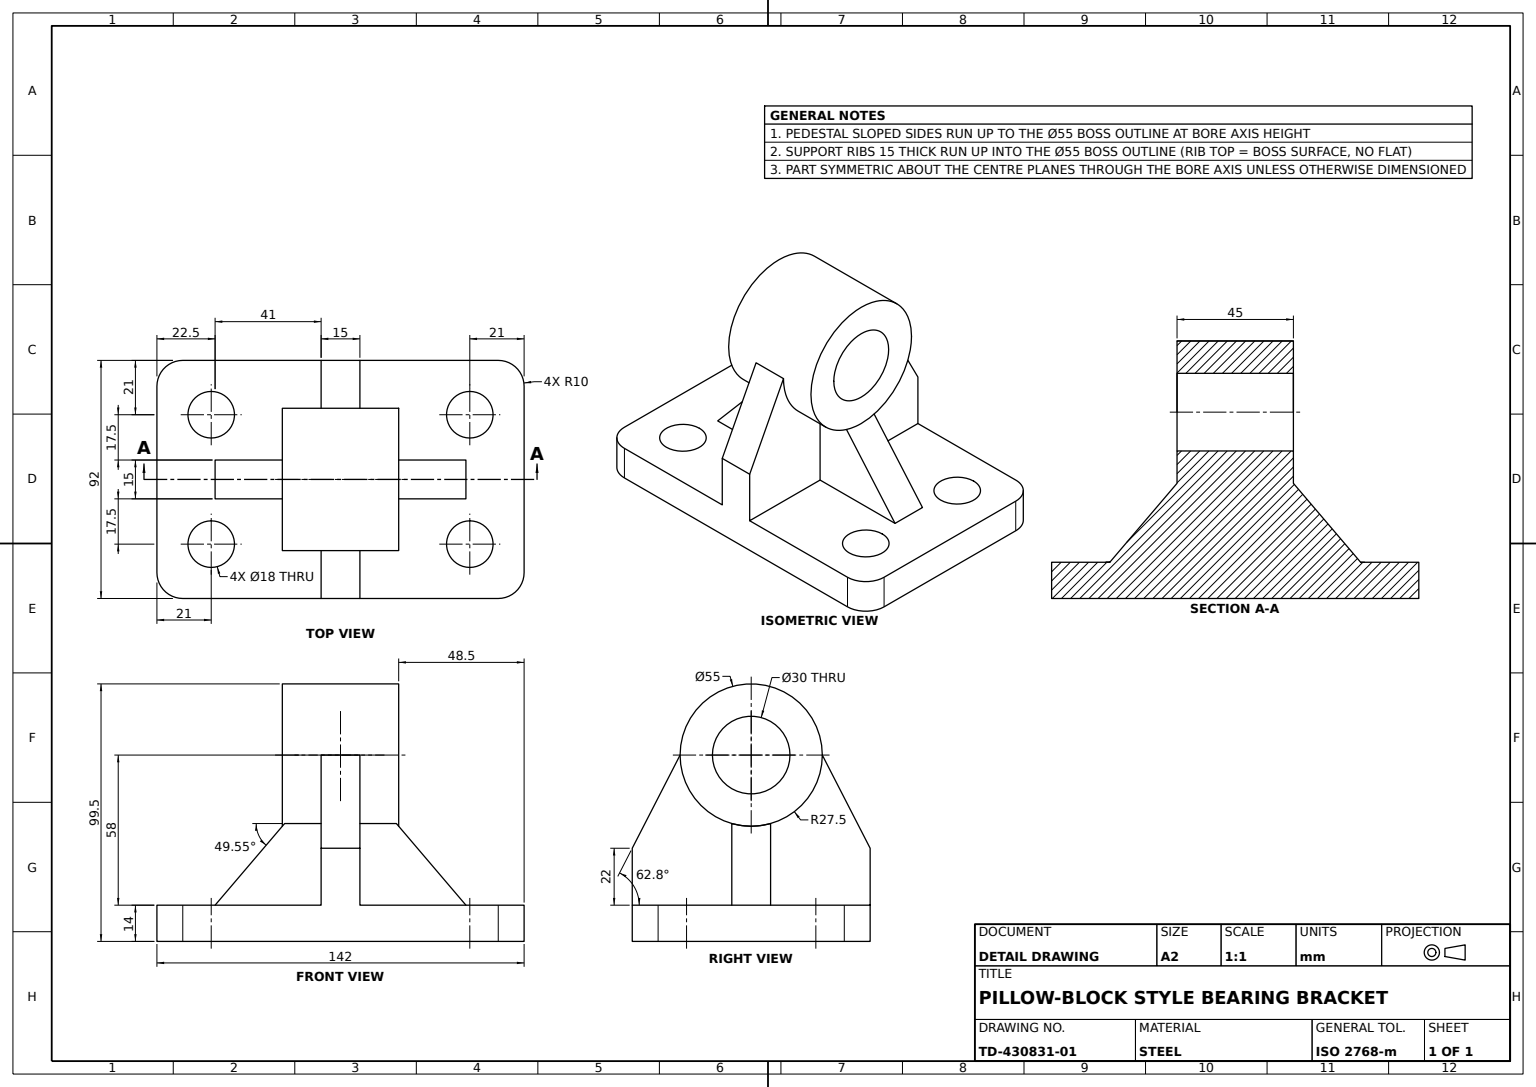
SolidWorks part; units mm, degrees
material "Plain Carbon Steel"
ref_plane "Front Plane" through (0, 0, 0) normal (0, 0, 1) x (1, 0, 0)
ref_plane "Top Plane" through (0, 0, 0) normal (0, 1, 0) x (1, 0, 0)
ref_plane "Right Plane" through (0, 0, 0) normal (1, 0, 0) x (0, 0, -1)
sketch "Base Plate Sketch" plane through (0, 0, 0) normal (0, 1, 0) x (1, 0, 0)
  line L1 (-71, -46) -> (71, -46)
  line L2 (-71, -46) -> (-71, 46)
  line L3 (-71, 46) -> (71, 46)
  line L4 (71, -46) -> (71, 46)
  line L5 (-71, -46) -> (71, 46) construction
  line L6 (-71, 46) -> (71, -46) construction
  point P0 (0, 0)
  dimension "D1" = 142
  dimension "D2" = 92
extrude "Base Plate 142x92x14" add sketch "Base Plate Sketch" along normal blind 14
fillet "Base Corner Fillets R10" radius 10 4 edges at (71, 7, -46) (-71, 7, -46) (-71, 7, 46) (71, 7, 46)
ref_plane "Plane1" through (0, 0, 0) normal (1, 0, 0) x (0, 0, -1)
sketch "Pedestal Sketch" plane through (0, 0, 0) normal (1, 0, 0) x (0, 0, -1)
  line L0 (46, 14) -> (46, 36)
  line L1 (-46, 14) -> (-46, 36)
  line L2 (-27.4995, 72) -> (27.5005, 72)
  line L3 (-36, 14) -> (36, 14) construction
  line L4 (-27.4995, 72) -> (-46, 36)
  line L5 (27.5005, 72) -> (46, 36)
  line L6 (-46, 14) -> (46, 14)
  point P9 (0.0005, 72)
  dimension "D1" = 22
  dimension "D2" = 22
  dimension "D3" = 27.4995
  dimension "D4" = 55
  dimension "D5" = 58
extrude "Bearing Pedestal" add sketch "Pedestal Sketch" along normal mid plane 15
ref_plane "Plane2" through (0, 0, 0) normal (0, 0, 1) x (1, 0, 0)
sketch "Bearing Boss Sketch" plane through (0, 0, 0) normal (1, 0, 0) x (0, 0, -1)
  line L0 (27.5005, 72) -> (-27.4995, 72) construction
  circle A0 centre (0.0005, 72) radius 27.5
  dimension "D1" = 55
extrude "Bearing Boss Ø55" add sketch "Bearing Boss Sketch" along normal mid plane 45
sketch "Bore Sketch" plane through (22.5, 0, 0) normal (1, 0, 0) x (0, 0, -1)
  circle A0 centre (0.0005, 72) radius 15
  dimension "D1" = 30
extrude "Bore Ø30" cut sketch "Bore Sketch" against normal through all
ref_plane "Plane3" through (0, 0, 0) normal (0, 0, 1) x (1, 0, 0)
sketch "Support Rib 1 Sketch" plane through (0, 0, 0) normal (0, 0, 1) x (1, 0, 0)
  line L0 (22.5, 44.5) -> (48.5, 14)
  line L1 (61, 14) -> (7.5, 14) construction
  line L2 (7.5, 14) -> (7.5, 36) construction
  dimension "D1" = 41
rib "Support Rib 1" sketch "Support Rib 1 Sketch" sketch "Support Rib 1 Sketch" thickness 15 extrusion direction parallel to sketch draft on no parameters "D1"=15
sketch "Support Rib 2 Sketch" plane through (0, 0, 0) normal (0, 0, 1) x (1, 0, 0)
  line L0 (-22.5, 44.5) -> (-48.5, 14)
  line L1 (-61, 14) -> (-7.5, 14) construction
  line L2 (-7.5, 36) -> (-7.5, 14) construction
  dimension "D1" = 41
rib "Support Rib 2" sketch "Support Rib 2 Sketch" sketch "Support Rib 2 Sketch" thickness 15 extrusion direction parallel to sketch draft on no parameters "D1"=15
sketch "Mounting Holes Sketch" plane through (0, 14, 0) normal (0, 1, 0) x (1, 0, 0)
  line L0 (-61, -46) -> (-7.5, -46) construction
  line L1 (7.5, -46) -> (61, -46) construction
  line L2 (61, 46) -> (7.5, 46) construction
  line L3 (-7.5, 46) -> (-61, 46) construction
  circle A0 centre (-50, 25) radius 9
  circle A1 centre (50, 25) radius 9
  circle A2 centre (50, -25) radius 9
  circle A3 centre (-50, -25) radius 9
  dimension "D1" = 18
  dimension "D2" = 18
  dimension "D3" = 18
  dimension "D4" = 18
  dimension "D5" = 21
  dimension "D6" = 21
  dimension "D7" = 21
  dimension "D8" = 21
  dimension "D9" = 27.5
  dimension "D10" = 27.5
  dimension "D11" = 27.5
  dimension "D12" = 27.5
extrude "Mounting Holes 4xØ18" cut sketch "Mounting Holes Sketch" against normal blind 41
